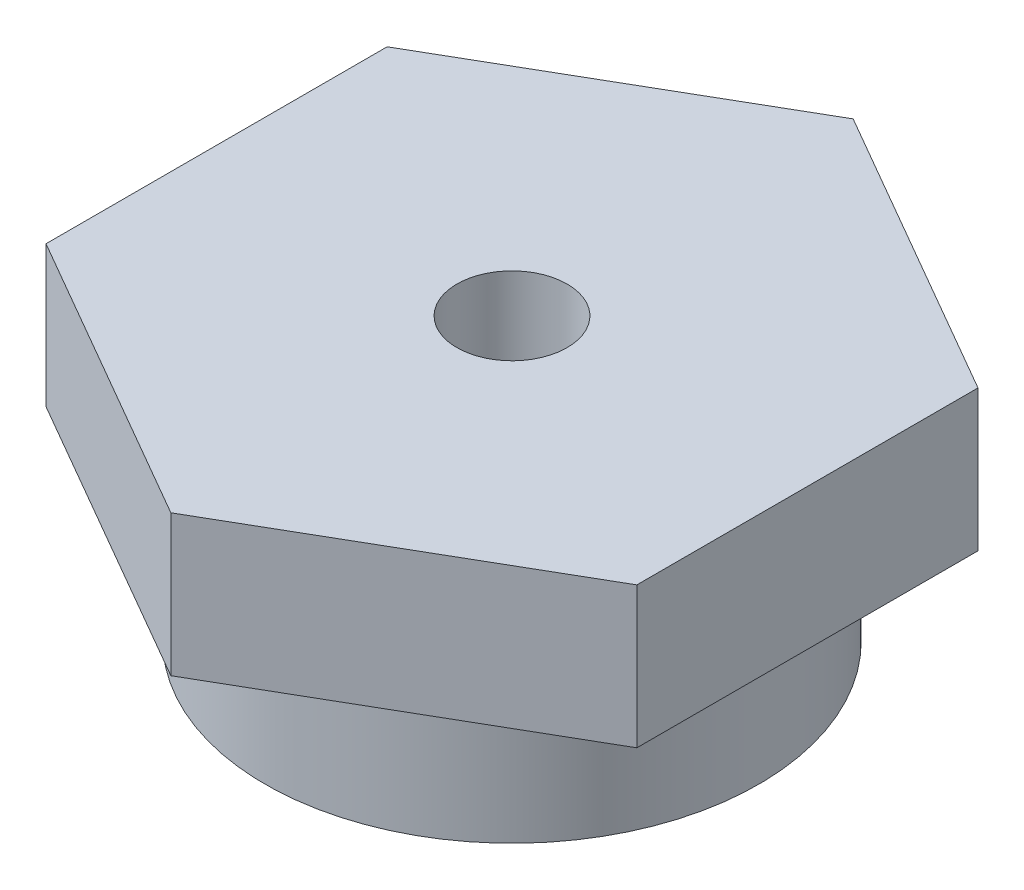
ISO-10303-21;
HEADER;
FILE_DESCRIPTION(('STEP AP214'),'2;1');
FILE_NAME('part.step','',(''),(''),'','','');
FILE_SCHEMA(('AUTOMOTIVE_DESIGN { 1 0 10303 214 1 1 1 1 }'));
ENDSEC;
DATA;
#1=APPLICATION_CONTEXT('core data for automotive mechanical design processes');
#2=APPLICATION_PROTOCOL_DEFINITION('international standard','automotive_design',2000,#1);
#3=PRODUCT_CONTEXT('',#1,'mechanical');
#4=PRODUCT('Part','Part','',(#3));
#5=PRODUCT_RELATED_PRODUCT_CATEGORY('part','',(#4));
#6=PRODUCT_DEFINITION_FORMATION('','',#4);
#7=PRODUCT_DEFINITION_CONTEXT('part definition',#1,'design');
#8=PRODUCT_DEFINITION('design','',#6,#7);
#9=PRODUCT_DEFINITION_SHAPE('','',#8);
#10=(LENGTH_UNIT() NAMED_UNIT(*) SI_UNIT(.MILLI.,.METRE.));
#11=(NAMED_UNIT(*) PLANE_ANGLE_UNIT() SI_UNIT($,.RADIAN.));
#12=(NAMED_UNIT(*) SI_UNIT($,.STERADIAN.) SOLID_ANGLE_UNIT());
#13=UNCERTAINTY_MEASURE_WITH_UNIT(LENGTH_MEASURE(1.E-05),#10,'distance_accuracy_value','');
#14=(GEOMETRIC_REPRESENTATION_CONTEXT(3) GLOBAL_UNCERTAINTY_ASSIGNED_CONTEXT((#13)) GLOBAL_UNIT_ASSIGNED_CONTEXT((#10,
#11,#12)) REPRESENTATION_CONTEXT('',''));
#15=CARTESIAN_POINT('',(0.,0.,0.));
#16=DIRECTION('',(0.,0.,1.));
#17=DIRECTION('',(1.,0.,0.));
#18=AXIS2_PLACEMENT_3D('',#15,#16,#17);
#19=CARTESIAN_POINT('',(-33.5,16.,19.3412340178525));
#20=DIRECTION('',(0.5,0.,-0.866025403784439));
#21=DIRECTION('',(-0.866025403784439,0.,-0.5));
#22=AXIS2_PLACEMENT_3D('',#19,#20,#21);
#23=PLANE('',#22);
#24=DIRECTION('',(0.866025403784438,0.,0.5));
#25=VECTOR('',#24,1.);
#26=CARTESIAN_POINT('',(-33.5,0.,19.3412340178525));
#27=LINE('',#26,#25);
#28=CARTESIAN_POINT('',(-33.5,0.,19.3412340178525));
#29=VERTEX_POINT('',#28);
#30=CARTESIAN_POINT('',(0.,0.,38.6824680357049));
#31=VERTEX_POINT('',#30);
#32=EDGE_CURVE('E125',#29,#31,#27,.T.);
#33=ORIENTED_EDGE('',*,*,#32,.T.);
#34=DIRECTION('',(0.,-1.,0.));
#35=VECTOR('',#34,1.);
#36=CARTESIAN_POINT('',(0.,16.,38.6824680357049));
#37=LINE('',#36,#35);
#38=CARTESIAN_POINT('',(0.,16.,38.6824680357049));
#39=VERTEX_POINT('',#38);
#40=EDGE_CURVE('E45',#39,#31,#37,.T.);
#41=ORIENTED_EDGE('',*,*,#40,.F.);
#42=DIRECTION('',(0.866025403784438,0.,0.5));
#43=VECTOR('',#42,1.);
#44=CARTESIAN_POINT('',(-33.5,16.,19.3412340178525));
#45=LINE('',#44,#43);
#46=CARTESIAN_POINT('',(-33.5,16.,19.3412340178525));
#47=VERTEX_POINT('',#46);
#48=EDGE_CURVE('E136',#47,#39,#45,.T.);
#49=ORIENTED_EDGE('',*,*,#48,.F.);
#50=DIRECTION('',(0.,-1.,0.));
#51=VECTOR('',#50,1.);
#52=CARTESIAN_POINT('',(-33.5,16.,19.3412340178525));
#53=LINE('',#52,#51);
#54=EDGE_CURVE('E121',#47,#29,#53,.T.);
#55=ORIENTED_EDGE('',*,*,#54,.T.);
#56=EDGE_LOOP('',(#33,#41,#49,#55));
#57=FACE_BOUND('',#56,.T.);
#58=ADVANCED_FACE('F39',(#57),#23,.F.);
#59=CARTESIAN_POINT('',(0.,16.,38.6824680357049));
#60=DIRECTION('',(-0.5,0.,-0.866025403784438));
#61=DIRECTION('',(-0.866025403784439,0.,0.5));
#62=AXIS2_PLACEMENT_3D('',#59,#60,#61);
#63=PLANE('',#62);
#64=DIRECTION('',(0.866025403784438,0.,-0.5));
#65=VECTOR('',#64,1.);
#66=CARTESIAN_POINT('',(0.,0.,38.6824680357049));
#67=LINE('',#66,#65);
#68=CARTESIAN_POINT('',(33.5,0.,19.3412340178525));
#69=VERTEX_POINT('',#68);
#70=EDGE_CURVE('E126',#31,#69,#67,.T.);
#71=ORIENTED_EDGE('',*,*,#70,.T.);
#72=DIRECTION('',(0.,-1.,0.));
#73=VECTOR('',#72,1.);
#74=CARTESIAN_POINT('',(33.5,16.,19.3412340178525));
#75=LINE('',#74,#73);
#76=CARTESIAN_POINT('',(33.5,16.,19.3412340178525));
#77=VERTEX_POINT('',#76);
#78=EDGE_CURVE('E138',#77,#69,#75,.T.);
#79=ORIENTED_EDGE('',*,*,#78,.F.);
#80=DIRECTION('',(0.866025403784438,0.,-0.5));
#81=VECTOR('',#80,1.);
#82=CARTESIAN_POINT('',(0.,16.,38.6824680357049));
#83=LINE('',#82,#81);
#84=EDGE_CURVE('E94',#39,#77,#83,.T.);
#85=ORIENTED_EDGE('',*,*,#84,.F.);
#86=ORIENTED_EDGE('',*,*,#40,.T.);
#87=EDGE_LOOP('',(#71,#79,#85,#86));
#88=FACE_BOUND('',#87,.T.);
#89=ADVANCED_FACE('F145',(#88),#63,.F.);
#90=CARTESIAN_POINT('',(33.5,16.,19.3412340178525));
#91=DIRECTION('',(-1.,0.,0.));
#92=DIRECTION('',(0.,0.,1.));
#93=AXIS2_PLACEMENT_3D('',#90,#91,#92);
#94=PLANE('',#93);
#95=DIRECTION('',(0.,0.,-1.));
#96=VECTOR('',#95,1.);
#97=CARTESIAN_POINT('',(33.5,0.,19.3412340178525));
#98=LINE('',#97,#96);
#99=CARTESIAN_POINT('',(33.5,0.,-19.3412340178525));
#100=VERTEX_POINT('',#99);
#101=EDGE_CURVE('E132',#69,#100,#98,.T.);
#102=ORIENTED_EDGE('',*,*,#101,.T.);
#103=DIRECTION('',(0.,-1.,0.));
#104=VECTOR('',#103,1.);
#105=CARTESIAN_POINT('',(33.5,16.,-19.3412340178525));
#106=LINE('',#105,#104);
#107=CARTESIAN_POINT('',(33.5,16.,-19.3412340178525));
#108=VERTEX_POINT('',#107);
#109=EDGE_CURVE('E117',#108,#100,#106,.T.);
#110=ORIENTED_EDGE('',*,*,#109,.F.);
#111=DIRECTION('',(0.,0.,-1.));
#112=VECTOR('',#111,1.);
#113=CARTESIAN_POINT('',(33.5,16.,19.3412340178525));
#114=LINE('',#113,#112);
#115=EDGE_CURVE('E110',#77,#108,#114,.T.);
#116=ORIENTED_EDGE('',*,*,#115,.F.);
#117=ORIENTED_EDGE('',*,*,#78,.T.);
#118=EDGE_LOOP('',(#102,#110,#116,#117));
#119=FACE_BOUND('',#118,.T.);
#120=ADVANCED_FACE('F147',(#119),#94,.F.);
#121=CARTESIAN_POINT('',(33.5,16.,-19.3412340178525));
#122=DIRECTION('',(-0.5,0.,0.866025403784439));
#123=DIRECTION('',(0.866025403784439,0.,0.5));
#124=AXIS2_PLACEMENT_3D('',#121,#122,#123);
#125=PLANE('',#124);
#126=DIRECTION('',(-0.866025403784439,0.,-0.5));
#127=VECTOR('',#126,1.);
#128=CARTESIAN_POINT('',(33.5,0.,-19.3412340178525));
#129=LINE('',#128,#127);
#130=CARTESIAN_POINT('',(0.,0.,-38.6824680357049));
#131=VERTEX_POINT('',#130);
#132=EDGE_CURVE('E113',#100,#131,#129,.T.);
#133=ORIENTED_EDGE('',*,*,#132,.T.);
#134=DIRECTION('',(0.,-1.,0.));
#135=VECTOR('',#134,1.);
#136=CARTESIAN_POINT('',(0.,16.,-38.6824680357049));
#137=LINE('',#136,#135);
#138=CARTESIAN_POINT('',(0.,16.,-38.6824680357049));
#139=VERTEX_POINT('',#138);
#140=EDGE_CURVE('E115',#139,#131,#137,.T.);
#141=ORIENTED_EDGE('',*,*,#140,.F.);
#142=DIRECTION('',(-0.866025403784439,0.,-0.5));
#143=VECTOR('',#142,1.);
#144=CARTESIAN_POINT('',(33.5,16.,-19.3412340178525));
#145=LINE('',#144,#143);
#146=EDGE_CURVE('E101',#108,#139,#145,.T.);
#147=ORIENTED_EDGE('',*,*,#146,.F.);
#148=ORIENTED_EDGE('',*,*,#109,.T.);
#149=EDGE_LOOP('',(#133,#141,#147,#148));
#150=FACE_BOUND('',#149,.T.);
#151=ADVANCED_FACE('F114',(#150),#125,.F.);
#152=CARTESIAN_POINT('',(0.,16.,-38.6824680357049));
#153=DIRECTION('',(0.5,0.,0.866025403784438));
#154=DIRECTION('',(0.866025403784438,0.,-0.5));
#155=AXIS2_PLACEMENT_3D('',#152,#153,#154);
#156=PLANE('',#155);
#157=DIRECTION('',(-0.866025403784438,0.,0.5));
#158=VECTOR('',#157,1.);
#159=CARTESIAN_POINT('',(0.,0.,-38.6824680357049));
#160=LINE('',#159,#158);
#161=CARTESIAN_POINT('',(-33.5,0.,-19.3412340178525));
#162=VERTEX_POINT('',#161);
#163=EDGE_CURVE('E76',#131,#162,#160,.T.);
#164=ORIENTED_EDGE('',*,*,#163,.T.);
#165=DIRECTION('',(0.,-1.,0.));
#166=VECTOR('',#165,1.);
#167=CARTESIAN_POINT('',(-33.5,16.,-19.3412340178525));
#168=LINE('',#167,#166);
#169=CARTESIAN_POINT('',(-33.5,16.,-19.3412340178525));
#170=VERTEX_POINT('',#169);
#171=EDGE_CURVE('E119',#170,#162,#168,.T.);
#172=ORIENTED_EDGE('',*,*,#171,.F.);
#173=DIRECTION('',(-0.866025403784438,0.,0.5));
#174=VECTOR('',#173,1.);
#175=CARTESIAN_POINT('',(0.,16.,-38.6824680357049));
#176=LINE('',#175,#174);
#177=EDGE_CURVE('E104',#139,#170,#176,.T.);
#178=ORIENTED_EDGE('',*,*,#177,.F.);
#179=ORIENTED_EDGE('',*,*,#140,.T.);
#180=EDGE_LOOP('',(#164,#172,#178,#179));
#181=FACE_BOUND('',#180,.T.);
#182=ADVANCED_FACE('F116',(#181),#156,.F.);
#183=CARTESIAN_POINT('',(-33.5,16.,-19.3412340178525));
#184=DIRECTION('',(1.,0.,0.));
#185=DIRECTION('',(0.,0.,-1.));
#186=AXIS2_PLACEMENT_3D('',#183,#184,#185);
#187=PLANE('',#186);
#188=DIRECTION('',(0.,0.,1.));
#189=VECTOR('',#188,1.);
#190=CARTESIAN_POINT('',(-33.5,0.,-19.3412340178525));
#191=LINE('',#190,#189);
#192=EDGE_CURVE('E85',#162,#29,#191,.T.);
#193=ORIENTED_EDGE('',*,*,#192,.T.);
#194=ORIENTED_EDGE('',*,*,#54,.F.);
#195=DIRECTION('',(0.,0.,1.));
#196=VECTOR('',#195,1.);
#197=CARTESIAN_POINT('',(-33.5,16.,-19.3412340178525));
#198=LINE('',#197,#196);
#199=EDGE_CURVE('E57',#170,#47,#198,.T.);
#200=ORIENTED_EDGE('',*,*,#199,.F.);
#201=ORIENTED_EDGE('',*,*,#171,.T.);
#202=EDGE_LOOP('',(#193,#194,#200,#201));
#203=FACE_BOUND('',#202,.T.);
#204=ADVANCED_FACE('F190',(#203),#187,.F.);
#205=CARTESIAN_POINT('',(0.,16.,0.));
#206=DIRECTION('',(0.,1.,0.));
#207=DIRECTION('',(0.,0.,1.));
#208=AXIS2_PLACEMENT_3D('',#205,#206,#207);
#209=PLANE('',#208);
#210=CARTESIAN_POINT('',(0.,16.,0.));
#211=DIRECTION('',(0.,-1.,0.));
#212=DIRECTION('',(0.,0.,-1.));
#213=AXIS2_PLACEMENT_3D('',#210,#211,#212);
#214=CIRCLE('',#213,6.25);
#215=CARTESIAN_POINT('',(0.,16.,-6.25));
#216=VERTEX_POINT('',#215);
#217=EDGE_CURVE('E156',#216,#216,#214,.T.);
#218=ORIENTED_EDGE('',*,*,#217,.T.);
#219=EDGE_LOOP('',(#218));
#220=FACE_BOUND('',#219,.T.);
#221=ORIENTED_EDGE('',*,*,#48,.T.);
#222=ORIENTED_EDGE('',*,*,#84,.T.);
#223=ORIENTED_EDGE('',*,*,#115,.T.);
#224=ORIENTED_EDGE('',*,*,#146,.T.);
#225=ORIENTED_EDGE('',*,*,#177,.T.);
#226=ORIENTED_EDGE('',*,*,#199,.T.);
#227=EDGE_LOOP('',(#221,#222,#223,#224,#225,#226));
#228=FACE_BOUND('',#227,.T.);
#229=ADVANCED_FACE('F103',(#220,#228),#209,.T.);
#230=CARTESIAN_POINT('',(0.,0.,0.));
#231=DIRECTION('',(0.,1.,0.));
#232=DIRECTION('',(0.,0.,1.));
#233=AXIS2_PLACEMENT_3D('',#230,#231,#232);
#234=PLANE('',#233);
#235=CARTESIAN_POINT('',(0.,0.,0.));
#236=DIRECTION('',(0.,-1.,0.));
#237=DIRECTION('',(0.,0.,-1.));
#238=AXIS2_PLACEMENT_3D('',#235,#236,#237);
#239=CIRCLE('',#238,28.);
#240=CARTESIAN_POINT('',(0.,0.,-28.));
#241=VERTEX_POINT('',#240);
#242=EDGE_CURVE('E11',#241,#241,#239,.T.);
#243=ORIENTED_EDGE('',*,*,#242,.F.);
#244=EDGE_LOOP('',(#243));
#245=FACE_BOUND('',#244,.T.);
#246=ORIENTED_EDGE('',*,*,#32,.F.);
#247=ORIENTED_EDGE('',*,*,#192,.F.);
#248=ORIENTED_EDGE('',*,*,#163,.F.);
#249=ORIENTED_EDGE('',*,*,#132,.F.);
#250=ORIENTED_EDGE('',*,*,#101,.F.);
#251=ORIENTED_EDGE('',*,*,#70,.F.);
#252=EDGE_LOOP('',(#246,#247,#248,#249,#250,#251));
#253=FACE_BOUND('',#252,.T.);
#254=ADVANCED_FACE('F149',(#245,#253),#234,.F.);
#255=CARTESIAN_POINT('',(0.,-16.,0.));
#256=DIRECTION('',(0.,1.,0.));
#257=DIRECTION('',(0.,0.,1.));
#258=AXIS2_PLACEMENT_3D('',#255,#256,#257);
#259=CYLINDRICAL_SURFACE('',#258,28.);
#260=CARTESIAN_POINT('',(0.,-16.,0.));
#261=DIRECTION('',(0.,-1.,0.));
#262=DIRECTION('',(0.,0.,-1.));
#263=AXIS2_PLACEMENT_3D('',#260,#261,#262);
#264=CIRCLE('',#263,28.);
#265=CARTESIAN_POINT('',(0.,-16.,-28.));
#266=VERTEX_POINT('',#265);
#267=EDGE_CURVE('E129',#266,#266,#264,.T.);
#268=ORIENTED_EDGE('',*,*,#267,.F.);
#269=EDGE_LOOP('',(#268));
#270=FACE_BOUND('',#269,.T.);
#271=ORIENTED_EDGE('',*,*,#242,.T.);
#272=EDGE_LOOP('',(#271));
#273=FACE_BOUND('',#272,.T.);
#274=ADVANCED_FACE('F175',(#270,#273),#259,.T.);
#275=CARTESIAN_POINT('',(0.,-16.,0.));
#276=DIRECTION('',(0.,-1.,0.));
#277=DIRECTION('',(0.,0.,-1.));
#278=AXIS2_PLACEMENT_3D('',#275,#276,#277);
#279=PLANE('',#278);
#280=CARTESIAN_POINT('',(0.,-16.,0.));
#281=DIRECTION('',(0.,-1.,0.));
#282=DIRECTION('',(0.,0.,-1.));
#283=AXIS2_PLACEMENT_3D('',#280,#281,#282);
#284=CIRCLE('',#283,6.25);
#285=CARTESIAN_POINT('',(0.,-16.,-6.25));
#286=VERTEX_POINT('',#285);
#287=EDGE_CURVE('E160',#286,#286,#284,.T.);
#288=ORIENTED_EDGE('',*,*,#287,.F.);
#289=EDGE_LOOP('',(#288));
#290=FACE_BOUND('',#289,.T.);
#291=ORIENTED_EDGE('',*,*,#267,.T.);
#292=EDGE_LOOP('',(#291));
#293=FACE_BOUND('',#292,.T.);
#294=ADVANCED_FACE('F170',(#290,#293),#279,.T.);
#295=CARTESIAN_POINT('',(0.,16.,0.));
#296=DIRECTION('',(0.,-1.,0.));
#297=DIRECTION('',(0.,0.,-1.));
#298=AXIS2_PLACEMENT_3D('',#295,#296,#297);
#299=CYLINDRICAL_SURFACE('',#298,6.25);
#300=ORIENTED_EDGE('',*,*,#217,.F.);
#301=EDGE_LOOP('',(#300));
#302=FACE_BOUND('',#301,.T.);
#303=ORIENTED_EDGE('',*,*,#287,.T.);
#304=EDGE_LOOP('',(#303));
#305=FACE_BOUND('',#304,.T.);
#306=ADVANCED_FACE('F163',(#302,#305),#299,.F.);
#307=CLOSED_SHELL('',(#58,#89,#120,#151,#182,#204,#229,#254,#274,#294,#306));
#308=MANIFOLD_SOLID_BREP('B2',#307);
#309=ADVANCED_BREP_SHAPE_REPRESENTATION('',(#18,#308),#14);
#310=SHAPE_DEFINITION_REPRESENTATION(#9,#309);
ENDSEC;
END-ISO-10303-21;
